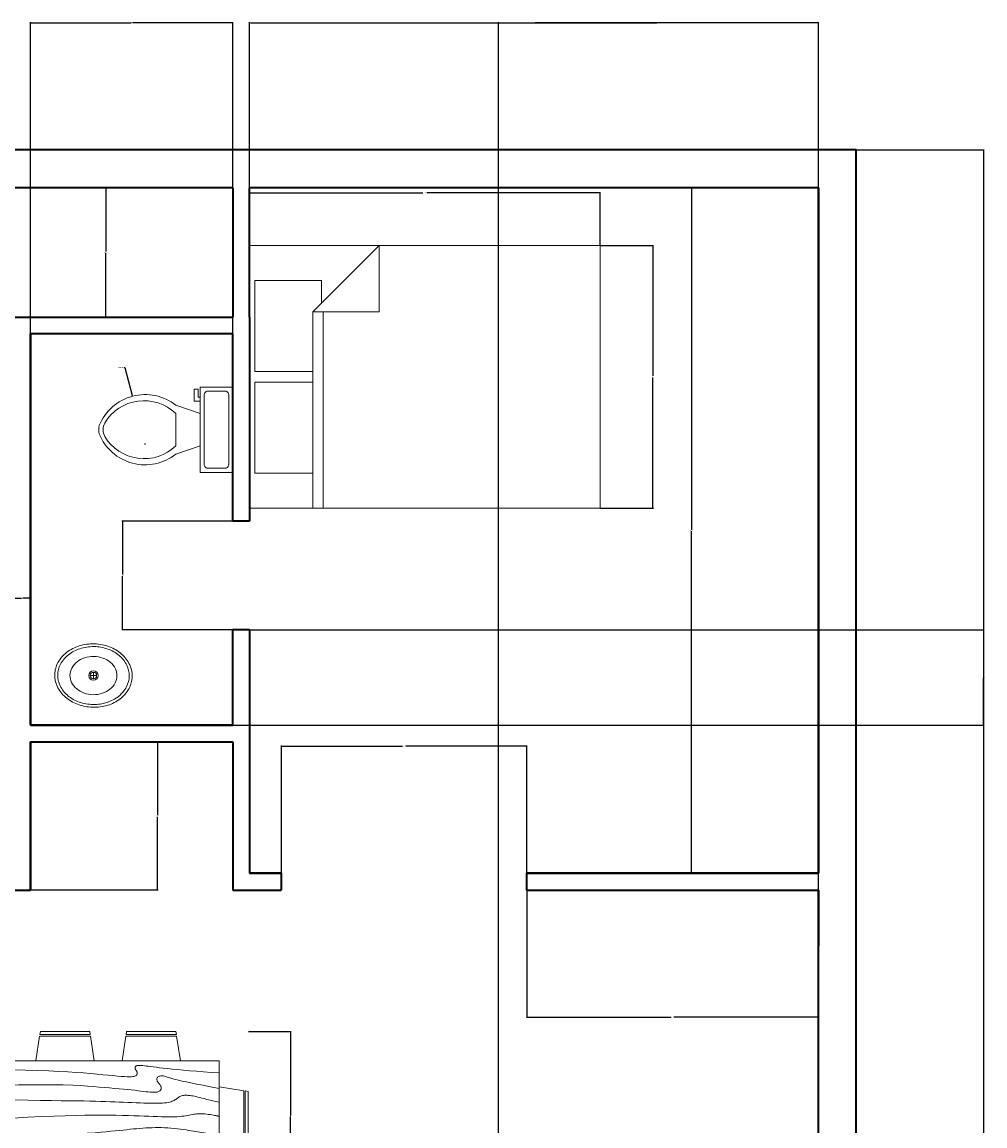
# Model space of a CAD drawing. Units: feet. Extents: x 2335 to 2876, y 491 to 1152.
# Tile 4 of 4: x 2648 to 2876, y 890 to 1152. Entities that reach past the tile are written whole.
import ezdxf

# ---------------------------------------------------------------- set-up
doc = ezdxf.new("R2010")
doc.units = ezdxf.units.FT
for name, color, linetype, lineweight in [('A-ANNO-DIMS', 2, 'Continuous', 18), ('A-FLOR-FIXT', 9, 'Continuous', 18), ('A-FURN', 8, 'Continuous', 18), ('A-WALL', 7, 'Continuous', 35), ('C-PROP', 3, 'Continuous', 35)]:
    doc.layers.add(name, color=color, linetype=linetype, lineweight=lineweight)
doc.styles.get("Standard").update_dxf_attribs({"font": 'arial.ttf'})
doc.dimstyles.get("Standard").update_dxf_attribs({"dimtxt": 0.18, "dimasz": 0.18, "dimexe": 0.18, "dimexo": 0.0625, "dimgap": 0.09, "dimtad": 0, "dimtih": 1, "dimtoh": 1, "dimdec": 4, "dimzin": 0, "dimdsep": 46, "dimlunit": 4, "dimtxsty": 'Standard', "dimcen": 0.09, "dimadec": 0, "dimazin": 0, "dimtfac": 1, "dimtdec": 4, "dimtofl": 0, "dimtmove": 0, "dimatfit": 3, "dimfxl": 1, "dimtolj": 1, "dimtzin": 0, "dimarcsym": 0})

# ---------------------------------------------------------------- blocks, each defined once
blk = doc.blocks.new('Bed - Queen')
for p, q in [((0, -80.00003), (0, 0)), ((0, 0), (59.99999, 0)), ((59.99999, 0), (59.99999, -80.00003)), ((7.99999, -1.2), (28.79998, -1.2)), ((7.99999, -14.4), (7.99999, -1.2)), ((28.79998, -1.2), (28.79998, -14.4)), ((31.19999, -1.2), (51.99999, -1.2)), ((31.19999, -14.4), (31.19999, -1.2)), ((51.99999, -1.2), (51.99999, -16.4)), ((0, -14.4), (44.8, -14.4)), ((59.99999, -29.6), (44.8, -14.4)), ((44.8, -14.4), (44.8, -29.6)), ((44.8, -16.8), (0, -16.8)), ((51.99999, -16.4), (46.79936, -16.4)), ((44.8, -29.6), (59.99999, -29.6)), ((59.99999, -80.00003), (0, -80.00003))]:
    blk.add_line(p, q)
blk = doc.blocks.new('Toilet - top')
for p, q in [((9.5, -6), (9.5, -2)), ((-8, -8.5), (-8, -8)), ((-7, -8), (-7, -9.5)), ((-4, -8), (-6, -14)), ((4, -8), (6, -14)), ((-10, -8.5), (-8, -8.5)), ((-10, -9.5), (-10, -8.5)), ((-7, -9.5), (-10, -9.5)), ((4, -14), (-4, -14))]:
    blk.add_line(p, q)
blk.add_lwpolyline([(10.5, -8), (10.5, 0), (-10.5, 0), (-10.5, -8)], close=True)
for points in [[(-9.5, -2), (-9.5, -6)], [(8.5, -1), (-8.5, -1)], [(-8.5, -7), (8.5, -7)]]:
    blk.add_lwpolyline(points)
for centre, radius, start, end in [((-8.62, -1.88), 0.884, 81.8699, 188.1301), ((8.62, -1.88), 0.884, 351.8699, 98.1301), ((-8.62, -6.12), 0.884, 171.8699, 278.1301), ((8.62, -6.12), 0.884, 261.8699, 8.1301), ((3.52, -21.58), 12.17, 141.4691, 247.9714), ((4.2, -21.82), 11.33, 136.3677, 238.9468), ((-3.52, -21.58), 12.17, 292.0284, 38.5307), ((-4.2, -21.82), 11.33, 301.053, 43.6321), ((0, -27.88), 4, 245.7318, 294.2682), ((0, -29), 4, 254.8605, 285.1395)]:
    blk.add_arc(centre, radius, start, end)
blk = doc.blocks.new('Sink - Oval top')
for p, q in [((-1, 0), (1, 0)), ((0, 1), (0, -1))]:
    blk.add_line(p, q)
for points in [[(-12.23, 0.39, 0.117634), (-11.46, -3.36, 0.104469), (-8.88, -6.8, 0.090016), (-5.08, -9.07, 0.08192), (-0.32, -10.02, 0.08192), (4.49, -9.38, 0.090016), (8.42, -7.36, 0.104469), (11.22, -4.09, 0.117634), (12.23, -0.39, 0.117634), (11.46, 3.36, 0.104469), (8.88, 6.8, 0.090016), (5.08, 9.07, 0.08192), (0.32, 10.02, 0.08192), (-4.49, 9.38, 0.090016), (-8.42, 7.36, 0.104469), (-11.22, 4.09, 0.117634)], [(-11.29, 0.16, 0.118622), (-10.52, -3.25, 0.104678), (-8.07, -6.36, 0.089562), (-4.54, -8.37, 0.081185), (-0.13, -9.15, 0.081185), (4.3, -8.49, 0.089562), (7.89, -6.58, 0.104678), (10.42, -3.55, 0.118622), (11.29, -0.16, 0.118622), (10.52, 3.25, 0.104678), (8.07, 6.36, 0.089562), (4.54, 8.37, 0.081185), (0.13, 9.15, 0.081185), (-4.3, 8.49, 0.089562), (-7.89, 6.58, 0.104678), (-10.42, 3.55, 0.118622)], [(-7.42, 0.08, 0.118283), (-6.91, -2.17, 0.104607), (-5.29, -4.21, 0.089718), (-2.97, -5.53, 0.081436), (-0.07, -6.04, 0.081436), (2.84, -5.59, 0.089718), (5.2, -4.33, 0.104607), (6.86, -2.32, 0.118283), (7.42, -0.08, 0.118283), (6.91, 2.17, 0.104607), (5.29, 4.21, 0.089718), (2.97, 5.53, 0.081436), (0.07, 6.04, 0.081436), (-2.84, 5.59, 0.089718), (-5.2, 4.33, 0.104607), (-6.86, 2.32, 0.118283)]]:
    blk.add_lwpolyline(points, format="xyb", close=True)
for radius in [1.5, 1]:
    blk.add_circle((0, 0), radius)
blk = doc.blocks.new('Dining Set - 36 x 72 in.')
for p, q in [((-22.2343, 26.00059), (-23.4847, 17.99762)), ((-22.2304, 26), (-5.7608, 26)), ((-22, 27.5), (-22.1562, 26.50042)), ((-5.8416, 26.5), (-22.1534, 26.5)), ((-22, 27.5), (-6, 27.5)), ((-5.8437, 26.49966), (-6, 27.5)), ((-4.5152, 17.99762), (-5.7655, 25.99926)), ((5.7657, 26.00059), (4.5153, 17.99762)), ((5.7696, 26), (22.2392, 26)), ((6, 27.5), (5.8438, 26.50042)), ((22.1584, 26.5), (5.8466, 26.5)), ((6, 27.5), (22, 27.5)), ((22.1563, 26.49966), (22, 27.5)), ((23.4848, 17.99762), (22.2345, 25.99926)), ((36, 18), (-36, 18)), ((-36, 18), (-36, -18)), ((36, -18), (36, 18)), ((-45.5, 8), (-44.5004, 8.15617)), ((-45.5, 8), (-45.5, -8)), ((-44.5, -8.15843), (-44.5, 8.15338)), ((-44.0006, 8.23428), (-35.9976, 9.48474)), ((-44, 8.23041), (-44, -8.23915)), ((44.0006, 8.23428), (35.9976, 9.48474)), ((44, 8.23041), (44, -8.23915)), ((44.5, -8.15843), (44.5, 8.15338)), ((45.5, 8), (44.5005, 8.15617)), ((45.5, 8), (45.5, -8)), ((-44.4997, -8.15631), (-45.5, -8)), ((-35.9976, -9.48476), (-43.9993, -8.2345)), ((35.9976, -9.48476), (43.9993, -8.2345)), ((44.4997, -8.15631), (45.5, -8)), ((-36, -18), (36, -18)), ((-22.2343, -26.0006), (-23.4847, -17.99762)), ((-4.5152, -17.99762), (-5.7655, -25.99928)), ((5.7657, -26.0006), (4.5153, -17.99762)), ((23.4848, -17.99762), (22.2345, -25.99928)), ((-22.2304, -26), (-5.7608, -26)), ((-22, -27.5), (-22.1562, -26.50044)), ((-5.8416, -26.5), (-22.1534, -26.5)), ((-22, -27.5), (-6, -27.5)), ((-5.8437, -26.49967), (-6, -27.5)), ((5.7696, -26), (22.2392, -26)), ((6, -27.5), (5.8438, -26.50044)), ((22.1584, -26.5), (5.8466, -26.5)), ((6, -27.5), (22, -27.5)), ((22.1563, -26.49967), (22, -27.5))]:
    blk.add_line(p, q)
for points in [[(-36, 15), (-31.1772, 14.97754), (-26.8079, 14.91406), (-22.8538, 14.81543), (-19.276, 14.6875), (-16.0362, 14.53613), (-13.0957, 14.36718), (-10.4159, 14.18652), (-7.9583, 14), (-5.6904, 13.81315), (-3.6035, 13.63021), (-1.6954, 13.45508), (0.0365, 13.29166), (1.5945, 13.14388), (2.9811, 13.01562), (4.1988, 12.9108), (5.25, 12.83333), (6.1393, 12.78613), (6.8802, 12.76823), (7.4883, 12.77767), (7.9792, 12.8125), (8.3685, 12.87077), (8.6719, 12.95052), (8.9049, 13.0498), (9.0833, 13.16666), (9.2205, 13.29899), (9.3216, 13.44401), (9.3895, 13.59879), (9.4271, 13.76041), (9.4373, 13.92594), (9.4232, 14.09245), (9.3875, 14.257), (9.3333, 14.41666), (9.2638, 14.56917), (9.1836, 14.71484), (9.0975, 14.85465), (9.0104, 14.98958), (8.9272, 15.1206), (8.8529, 15.2487), (8.7922, 15.37483), (8.75, 15.5), (8.7305, 15.62467), (8.7344, 15.74739), (8.7617, 15.86621), (8.8125, 15.97916), (8.8867, 16.08431), (8.9844, 16.17968), (9.1055, 16.26334), (9.25, 16.33333), (9.4189, 16.38802), (9.6172, 16.42708), (9.8506, 16.45052), (10.125, 16.45833), (10.4463, 16.45052), (10.8203, 16.42708), (11.2529, 16.38802), (11.75, 16.33333), (12.3184, 16.26318), (12.9694, 16.17838), (13.7151, 16.07991), (14.5677, 15.96875), (15.5395, 15.84586), (16.6426, 15.71224), (17.8893, 15.56884), (19.2917, 15.41666), (20.859, 15.25667), (22.5879, 15.08984), (24.4721, 14.91715), (26.5052, 14.73958), (28.6809, 14.5581), (30.9929, 14.3737), (33.4347, 14.18733), (36, 14)], [(-36, 10), (-28.9766, 10.14274), (-23.1725, 10.20442), (-18.4241, 10.19775), (-14.5677, 10.13541), (-11.4399, 10.03011), (-8.877, 9.89453), (-6.7154, 9.74137), (-4.7917, 9.58333), (-2.9698, 9.43082), (-1.2246, 9.28515), (0.4415, 9.14534), (2.026, 9.01041), (3.5266, 8.87939), (4.9408, 8.7513), (6.266, 8.62516), (7.5, 8.5), (8.6411, 8.37549), (9.6914, 8.2539), (10.6538, 8.13818), (11.5312, 8.03125), (12.3267, 7.93603), (13.043, 7.85547), (13.6831, 7.79248), (14.25, 7.75), (14.7471, 7.7303), (15.1797, 7.73307), (15.5537, 7.75732), (15.875, 7.80208), (16.1494, 7.86637), (16.3828, 7.94922), (16.5811, 8.04964), (16.75, 8.16666), (16.8944, 8.29915), (17.0143, 8.44531), (17.1089, 8.60319), (17.1771, 8.77083), (17.218, 8.94629), (17.2305, 9.1276), (17.2137, 9.31282), (17.1667, 9.5), (17.0895, 9.6875), (16.987, 9.875), (16.8649, 10.0625), (16.7292, 10.25), (16.5856, 10.4375), (16.4401, 10.625), (16.2985, 10.8125), (16.1667, 11), (16.05, 11.18733), (15.9518, 11.3737), (15.8752, 11.5581), (15.8229, 11.73958), (15.798, 11.91715), (15.8034, 12.08984), (15.842, 12.25667), (15.9167, 12.41666), (16.0295, 12.56836), (16.1784, 12.70833), (16.3605, 12.83268), (16.5729, 12.9375), (16.8127, 13.01888), (17.0768, 13.07291), (17.3625, 13.0957), (17.6667, 13.08333), (17.9894, 13.03312), (18.3418, 12.94726), (18.7382, 12.82918), (19.1927, 12.68229), (19.7195, 12.51001), (20.3327, 12.31575), (21.0465, 12.10294), (21.875, 11.875), (22.8357, 11.63354), (23.959, 11.37304), (25.2786, 11.08618), (26.8282, 10.76562), (28.6414, 10.40405), (30.752, 9.99414), (33.1936, 9.52856), (36, 9)], [(-36, 5.5), (-30.7157, 5.3348), (-26.069, 5.20963), (-21.9946, 5.11767), (-18.4271, 5.05208), (-15.3009, 5.00602), (-12.5508, 4.97265), (-10.1112, 4.94515), (-7.9167, 4.91666), (-5.909, 4.88167), (-4.0586, 4.83984), (-2.3429, 4.79215), (-0.7396, 4.73958), (0.7739, 4.6831), (2.22, 4.6237), (3.6213, 4.56233), (5, 4.5), (6.373, 4.43782), (7.7344, 4.3776), (9.0723, 4.32129), (10.375, 4.27083), (11.6309, 4.22819), (12.8281, 4.19531), (13.9551, 4.17415), (15, 4.16666), (15.954, 4.17448), (16.819, 4.19791), (17.6001, 4.23698), (18.3021, 4.29166), (18.9299, 4.36198), (19.4883, 4.44791), (19.9823, 4.54948), (20.4167, 4.66666), (20.7969, 4.79899), (21.1302, 4.94401), (21.4245, 5.09879), (21.6875, 5.26041), (21.9271, 5.42594), (22.1511, 5.59245), (22.3672, 5.757), (22.5834, 5.91666), (22.8065, 6.06868), (23.0404, 6.21093), (23.2879, 6.34147), (23.5521, 6.45833), (23.8358, 6.55957), (24.142, 6.64323), (24.4735, 6.70735), (24.8334, 6.75), (25.2235, 6.76969), (25.642, 6.76692), (26.0858, 6.74267), (26.5521, 6.69791), (27.0379, 6.63362), (27.5404, 6.55078), (28.0565, 6.45036), (28.5834, 6.33333), (29.1242, 6.19987), (29.7071, 6.04687), (30.3661, 5.87044), (31.1354, 5.66666), (32.0493, 5.43164), (33.142, 5.16146), (34.4475, 4.85221), (36, 4.5)], [(-36, -1), (-30.7915, -0.6591), (-26.0195, -0.38216), (-21.6519, -0.16284), (-17.6563, 0.00521), (-14.0005, 0.12833), (-10.6523, 0.21289), (-7.5796, 0.26522), (-4.75, 0.29166), (-2.134, 0.29793), (0.2878, 0.28711), (2.5317, 0.26163), (4.6146, 0.22396), (6.5529, 0.17651), (8.3633, 0.12174), (10.0623, 0.06209), (11.6667, 0), (13.1899, -0.06201), (14.6341, -0.1211), (15.9982, -0.17432), (17.2813, -0.21875), (18.4823, -0.25147), (19.6003, -0.26953), (20.6343, -0.27002), (21.5834, -0.25), (22.4481, -0.20768), (23.2357, -0.14584), (23.9549, -0.06836), (24.6146, 0.02083), (25.2235, 0.11784), (25.7904, 0.21875), (26.3241, 0.31966), (26.8334, 0.41666), (27.3265, 0.50618), (27.8099, 0.58593), (28.2894, 0.65397), (28.7709, 0.70833), (29.2601, 0.74707), (29.763, 0.76823), (30.2855, 0.76985), (30.8334, 0.75), (31.4088, 0.70784), (31.9994, 0.64713), (32.589, 0.57275), (33.1615, 0.48958), (33.7008, 0.4025), (34.1908, 0.3164), (34.6153, 0.23616), (34.9584, 0.16666), (35.2099, 0.11165), (35.3848, 0.07031), (35.504, 0.04069), (35.5886, 0.02083), (35.6594, 0.00879), (35.7377, 0.0026), (35.8442, 0.00032), (36, 0)], [(-36, -6.5), (-27.1843, -6.31267), (-20.084, -6.1263), (-14.469, -5.9419), (-10.1094, -5.76042), (-6.7752, -5.58285), (-4.2363, -5.41016), (-2.2629, -5.24333), (-0.625, -5.08334), (0.8708, -4.93099), (2.2715, -4.78646), (3.5872, -4.64974), (4.8281, -4.52084), (6.0046, -4.39974), (7.127, -4.28646), (8.2053, -4.18099), (9.25, -4.08334), (10.2705, -3.99382), (11.2734, -3.91407), (12.2647, -3.84603), (13.25, -3.79167), (14.2354, -3.75293), (15.2266, -3.73177), (16.2295, -3.73015), (17.25, -3.75), (18.2912, -3.79248), (19.3451, -3.85547), (20.4009, -3.93604), (21.4479, -4.03125), (22.4754, -4.13819), (23.4727, -4.25391), (24.4289, -4.37549), (25.3334, -4.5), (26.1785, -4.62492), (26.9694, -4.74935), (27.7145, -4.87281), (28.4219, -4.99479), (29.1, -5.11483), (29.7572, -5.23242), (30.4016, -5.34709), (31.0417, -5.45834), (31.6837, -5.56437), (32.3262, -5.65821), (32.9658, -5.73153), (33.599, -5.77604), (34.2224, -5.78345), (34.8327, -5.74545), (35.4264, -5.65373), (36, -5.5)], [(-36, -10), (-26.4022, -9.81299), (-18.4675, -9.62891), (-11.9839, -9.45069), (-6.7396, -9.28125), (-2.5226, -9.12354), (0.8789, -8.98047), (3.6769, -8.85498), (6.0833, -8.75), (8.2767, -8.66765), (10.3021, -8.60677), (12.1712, -8.56543), (13.8958, -8.54167), (15.4876, -8.53353), (16.9583, -8.53907), (18.3197, -8.55632), (19.5834, -8.58334), (20.7616, -8.61841), (21.8685, -8.66081), (22.9188, -8.71004), (23.9271, -8.76563), (24.9081, -8.82707), (25.8763, -8.89388), (26.8465, -8.96558), (27.8334, -9.04167), (28.8474, -9.12118), (29.8828, -9.20117), (30.93, -9.27824), (31.9792, -9.34896), (33.0205, -9.40991), (34.0443, -9.45768), (35.0407, -9.48885), (36, -9.5)], [(-36, -14.5), (-30.0881, -14.33513), (-25.0332, -14.21224), (-20.7312, -14.12647), (-17.0781, -14.07292), (-13.97, -14.04671), (-11.3027, -14.04297), (-8.9724, -14.05681), (-6.875, -14.08334), (-4.9224, -14.11833), (-3.0905, -14.16016), (-1.3709, -14.20785), (0.2448, -14.26042), (1.7647, -14.3169), (3.1973, -14.3763), (4.5507, -14.43767), (5.8333, -14.5), (7.0554, -14.5621), (8.235, -14.62175), (9.3922, -14.67652), (10.5469, -14.72396), (11.7192, -14.76164), (12.929, -14.78711), (14.1965, -14.79794), (15.5417, -14.79167), (16.9933, -14.76424), (18.6152, -14.70508), (20.4804, -14.60197), (22.6615, -14.44271), (25.2312, -14.21509), (28.2624, -13.9069), (31.8277, -13.50594), (36, -13)]]:
    blk.add_lwpolyline(points)
blk = doc.blocks.new('*D10')
at = {"layer": 'A-ANNO-DIMS', "color": 0, "lineweight": -2, "transparency": 16777216}
for p, q in [((2701.8, 1098.88), (2701.8, 1111.48)), ((2701.98, 1111.3), (2742.89, 1111.3)), ((2784.81, 1111.3), (2743.9, 1111.3)), ((2784.99, 1098.88), (2784.99, 1111.48))]:
    blk.add_line(p, q, dxfattribs=at)
at = {"layer": 'A-ANNO-DIMS', "color": 0, "transparency": 16777216}
for points in [[(2701.98, 1111.33), (2701.98, 1111.27), (2701.8, 1111.3)], [(2784.81, 1111.33), (2784.81, 1111.27), (2784.99, 1111.3)]]:
    blk.add_solid(points, dxfattribs=at)
at = {"layer": 'Defpoints', "color": 0, "transparency": 16777216}
for p in [(2701.8, 1111.3), (2701.8, 1098.82), (2784.99, 1098.82)]:
    blk.add_point(p, dxfattribs=at)
at = {"layer": 'A-ANNO-DIMS', "color": 0, "transparency": 16777216, "insert": (2743.4, 1111.3), "char_height": 0.18, "attachment_point": 5}
blk.add_mtext('\\A1;BED 83', dxfattribs=at)
blk = doc.blocks.new('*D11')
at = {"layer": 'A-ANNO-DIMS', "color": 0, "lineweight": -2, "transparency": 16777216}
for p, q in [((2785.06, 1098.82), (2797.65, 1098.82)), ((2797.47, 1098.64), (2797.47, 1067.81)), ((2797.47, 1036.6), (2797.47, 1067.44)), ((2785.06, 1036.42), (2797.65, 1036.42))]:
    blk.add_line(p, q, dxfattribs=at)
at = {"layer": 'A-ANNO-DIMS', "color": 0, "transparency": 16777216}
for points in [[(2797.44, 1098.64), (2797.5, 1098.64), (2797.47, 1098.82)], [(2797.44, 1036.6), (2797.5, 1036.6), (2797.47, 1036.42)]]:
    blk.add_solid(points, dxfattribs=at)
at = {"layer": 'Defpoints', "color": 0, "transparency": 16777216}
for p in [(2784.99, 1098.82), (2797.47, 1098.82), (2784.99, 1036.42)]:
    blk.add_point(p, dxfattribs=at)
at = {"layer": 'A-ANNO-DIMS', "color": 0, "transparency": 16777216, "insert": (2797.47, 1067.62), "char_height": 0.18, "attachment_point": 5}
blk.add_mtext('\\A1;62', dxfattribs=at)
blk = doc.blocks.new('*D21')
at = {"layer": 'A-ANNO-DIMS', "color": 0, "lineweight": -2, "transparency": 16777216}
for p, q in [((2701.56, 912.23), (2711.65, 912.23)), ((2711.47, 912.05), (2711.47, 892.31)), ((2711.47, 872.2), (2711.47, 891.94)), ((2701.56, 872.02), (2711.65, 872.02))]:
    blk.add_line(p, q, dxfattribs=at)
at = {"layer": 'A-ANNO-DIMS', "color": 0, "transparency": 16777216}
for points in [[(2711.44, 912.05), (2711.5, 912.05), (2711.47, 912.23)], [(2711.44, 872.2), (2711.5, 872.2), (2711.47, 872.02)]]:
    blk.add_solid(points, dxfattribs=at)
at = {"layer": 'Defpoints', "color": 0, "transparency": 16777216}
for p in [(2701.49, 912.23), (2711.47, 912.23), (2701.49, 872.02)]:
    blk.add_point(p, dxfattribs=at)
at = {"layer": 'A-ANNO-DIMS', "color": 0, "transparency": 16777216, "insert": (2711.47, 892.13), "char_height": 0.18, "attachment_point": 5}
blk.add_mtext('\\A1;40', dxfattribs=at)
blk = doc.blocks.new('*D25')
at = {"layer": 'A-ANNO-DIMS', "color": 0, "lineweight": -2, "transparency": 16777216}
for p, q in [((2845.86, 1121.49), (2876.13, 1121.49)), ((2875.95, 1121.31), (2875.95, 821.67)), ((2875.95, 521.67), (2875.95, 821.31)), ((2845.86, 521.49), (2876.13, 521.49))]:
    blk.add_line(p, q, dxfattribs=at)
at = {"layer": 'A-ANNO-DIMS', "color": 0, "transparency": 16777216}
for points in [[(2875.92, 1121.31), (2875.98, 1121.31), (2875.95, 1121.49)], [(2875.92, 521.67), (2875.98, 521.67), (2875.95, 521.49)]]:
    blk.add_solid(points, dxfattribs=at)
at = {"layer": 'Defpoints', "color": 0, "transparency": 16777216}
for p in [(2845.8, 1121.49), (2875.95, 1121.49), (2845.8, 521.49)]:
    blk.add_point(p, dxfattribs=at)
at = {"layer": 'A-ANNO-DIMS', "color": 0, "transparency": 16777216, "insert": (2875.95, 821.49), "char_height": 0.18, "attachment_point": 5}
blk.add_mtext('\\A1;600', dxfattribs=at)
blk = doc.blocks.new('*D36')
at = {"layer": 'A-ANNO-DIMS', "color": 0, "lineweight": -2, "transparency": 16777216}
for p, q in [((2836.73, 1112.49), (2806.47, 1112.49)), ((2806.65, 1112.31), (2806.65, 1031.32)), ((2806.65, 949.98), (2806.65, 1030.96)), ((2836.73, 949.8), (2806.47, 949.8))]:
    blk.add_line(p, q, dxfattribs=at)
at = {"layer": 'A-ANNO-DIMS', "color": 0, "transparency": 16777216}
for points in [[(2806.62, 1112.31), (2806.68, 1112.31), (2806.65, 1112.49)], [(2806.62, 949.98), (2806.68, 949.98), (2806.65, 949.8)]]:
    blk.add_solid(points, dxfattribs=at)
at = {"layer": 'Defpoints', "color": 0, "transparency": 16777216}
for p in [(2806.65, 1112.49), (2836.8, 1112.49), (2836.8, 949.8)]:
    blk.add_point(p, dxfattribs=at)
at = {"layer": 'A-ANNO-DIMS', "color": 0, "transparency": 16777216, "insert": (2806.65, 1031.14), "char_height": 0.18, "attachment_point": 5}
blk.add_mtext('\\A1;162.7', dxfattribs=at)
blk = doc.blocks.new('*D37')
at = {"layer": 'A-ANNO-DIMS', "color": 0, "lineweight": -2, "transparency": 16777216}
for p, q in [((2760.88, 882.29), (2760.88, 1151.82)), ((2761.06, 1151.64), (2798.45, 1151.64)), ((2836.62, 1151.64), (2799.23, 1151.64)), ((2836.8, 882.29), (2836.8, 1151.82))]:
    blk.add_line(p, q, dxfattribs=at)
at = {"layer": 'A-ANNO-DIMS', "color": 0, "transparency": 16777216}
for points in [[(2761.06, 1151.67), (2761.06, 1151.61), (2760.88, 1151.64)], [(2836.62, 1151.67), (2836.62, 1151.61), (2836.8, 1151.64)]]:
    blk.add_solid(points, dxfattribs=at)
at = {"layer": 'Defpoints', "color": 0, "transparency": 16777216}
for p in [(2836.8, 1151.64), (2760.88, 882.23), (2836.8, 882.23)]:
    blk.add_point(p, dxfattribs=at)
at = {"layer": 'A-ANNO-DIMS', "color": 0, "transparency": 16777216, "insert": (2798.84, 1151.64), "char_height": 0.18, "attachment_point": 5}
blk.add_mtext('\\A1;75.92', dxfattribs=at)
blk = doc.blocks.new('*D56')
at = {"layer": 'A-ANNO-DIMS', "color": 0, "lineweight": -2, "transparency": 16777216}
for p, q in [((2649.8, 1077.86), (2649.8, 1151.82)), ((2649.98, 1151.64), (2673.57, 1151.64)), ((2697.62, 1151.64), (2674.02, 1151.64)), ((2697.8, 1077.86), (2697.8, 1151.82))]:
    blk.add_line(p, q, dxfattribs=at)
at = {"layer": 'A-ANNO-DIMS', "color": 0, "transparency": 16777216}
for points in [[(2649.98, 1151.67), (2649.98, 1151.61), (2649.8, 1151.64)], [(2697.62, 1151.67), (2697.62, 1151.61), (2697.8, 1151.64)]]:
    blk.add_solid(points, dxfattribs=at)
at = {"layer": 'Defpoints', "color": 0, "transparency": 16777216}
for p in [(2697.8, 1151.64), (2649.8, 1077.8), (2697.8, 1077.8)]:
    blk.add_point(p, dxfattribs=at)
at = {"layer": 'A-ANNO-DIMS', "color": 0, "transparency": 16777216, "insert": (2673.8, 1151.64), "char_height": 0.18, "attachment_point": 5}
blk.add_mtext('\\A1;48', dxfattribs=at)
blk = doc.blocks.new('*D57')
at = {"layer": 'A-ANNO-DIMS', "color": 0, "lineweight": -2, "transparency": 16777216}
for p, q in [((2645.8, 985.02), (2645.8, 1015.28)), ((2645.98, 1015.1), (2647.65, 1015.1)), ((2649.62, 1015.1), (2647.95, 1015.1)), ((2649.8, 985.02), (2649.8, 1015.28))]:
    blk.add_line(p, q, dxfattribs=at)
at = {"layer": 'A-ANNO-DIMS', "color": 0, "transparency": 16777216}
for points in [[(2645.98, 1015.13), (2645.98, 1015.07), (2645.8, 1015.1)], [(2649.62, 1015.13), (2649.62, 1015.07), (2649.8, 1015.1)]]:
    blk.add_solid(points, dxfattribs=at)
at = {"layer": 'Defpoints', "color": 0, "transparency": 16777216}
for p in [(2649.8, 1015.1), (2645.8, 984.95), (2649.8, 984.95)]:
    blk.add_point(p, dxfattribs=at)
at = {"layer": 'A-ANNO-DIMS', "color": 0, "transparency": 16777216, "insert": (2647.8, 1015.1), "char_height": 0.18, "attachment_point": 5}
blk.add_mtext('\\A1;4', dxfattribs=at)
blk = doc.blocks.new('*D59')
at = {"layer": 'A-ANNO-DIMS', "color": 0, "lineweight": -2, "transparency": 16777216}
for p, q in [((2649.86, 980.95), (2680.13, 980.95)), ((2679.95, 980.77), (2679.95, 963.56)), ((2679.95, 945.98), (2679.95, 963.19)), ((2649.86, 945.8), (2680.13, 945.8))]:
    blk.add_line(p, q, dxfattribs=at)
at = {"layer": 'A-ANNO-DIMS', "color": 0, "transparency": 16777216}
for points in [[(2679.92, 980.77), (2679.98, 980.77), (2679.95, 980.95)], [(2679.92, 945.98), (2679.98, 945.98), (2679.95, 945.8)]]:
    blk.add_solid(points, dxfattribs=at)
at = {"layer": 'Defpoints', "color": 0, "transparency": 16777216}
for p in [(2649.8, 980.95), (2649.8, 945.8), (2679.95, 945.8)]:
    blk.add_point(p, dxfattribs=at)
at = {"layer": 'A-ANNO-DIMS', "color": 0, "transparency": 16777216, "insert": (2679.95, 963.38), "char_height": 0.18, "attachment_point": 5}
blk.add_mtext('\\A1;35.155', dxfattribs=at)
blk = doc.blocks.new('*D60')
at = {"layer": 'A-ANNO-DIMS', "color": 0, "lineweight": -2, "transparency": 16777216}
for p, q in [((2697.73, 1112.49), (2667.47, 1112.49)), ((2667.65, 1112.31), (2667.65, 1097.32)), ((2667.65, 1081.98), (2667.65, 1096.96)), ((2697.73, 1081.8), (2667.47, 1081.8))]:
    blk.add_line(p, q, dxfattribs=at)
at = {"layer": 'A-ANNO-DIMS', "color": 0, "transparency": 16777216}
for points in [[(2667.62, 1112.31), (2667.68, 1112.31), (2667.65, 1112.49)], [(2667.62, 1081.98), (2667.68, 1081.98), (2667.65, 1081.8)]]:
    blk.add_solid(points, dxfattribs=at)
at = {"layer": 'Defpoints', "color": 0, "transparency": 16777216}
for p in [(2667.65, 1112.49), (2697.8, 1112.49), (2697.8, 1081.8)]:
    blk.add_point(p, dxfattribs=at)
at = {"layer": 'A-ANNO-DIMS', "color": 0, "transparency": 16777216, "insert": (2667.65, 1097.14), "char_height": 0.18, "attachment_point": 5}
blk.add_mtext('\\A1;30.69', dxfattribs=at)
blk = doc.blocks.new('*D61')
at = {"layer": 'A-ANNO-DIMS', "color": 0, "lineweight": -2, "transparency": 16777216}
for p, q in [((2701.8, 1112.55), (2701.8, 1151.82)), ((2701.98, 1151.64), (2769.02, 1151.64)), ((2836.62, 1151.64), (2769.58, 1151.64)), ((2836.8, 1112.55), (2836.8, 1151.82))]:
    blk.add_line(p, q, dxfattribs=at)
at = {"layer": 'A-ANNO-DIMS', "color": 0, "transparency": 16777216}
for points in [[(2701.98, 1151.67), (2701.98, 1151.61), (2701.8, 1151.64)], [(2836.62, 1151.67), (2836.62, 1151.61), (2836.8, 1151.64)]]:
    blk.add_solid(points, dxfattribs=at)
at = {"layer": 'Defpoints', "color": 0, "transparency": 16777216}
for p in [(2836.8, 1151.64), (2701.8, 1112.49), (2836.8, 1112.49)]:
    blk.add_point(p, dxfattribs=at)
at = {"layer": 'A-ANNO-DIMS', "color": 0, "transparency": 16777216, "insert": (2769.3, 1151.64), "char_height": 0.18, "attachment_point": 5}
blk.add_mtext('\\A1;135', dxfattribs=at)
blk = doc.blocks.new('*D62')
at = {"layer": 'A-ANNO-DIMS', "color": 0, "lineweight": -2, "transparency": 16777216}
for p, q in [((2709.33, 949.86), (2709.33, 980.13)), ((2767.62, 949.86), (2767.62, 980.13)), ((2709.51, 979.95), (2738.08, 979.95)), ((2767.44, 979.95), (2738.87, 979.95))]:
    blk.add_line(p, q, dxfattribs=at)
at = {"layer": 'A-ANNO-DIMS', "color": 0, "transparency": 16777216}
for points in [[(2709.51, 979.98), (2709.51, 979.92), (2709.33, 979.95)], [(2767.44, 979.98), (2767.44, 979.92), (2767.62, 979.95)]]:
    blk.add_solid(points, dxfattribs=at)
at = {"layer": 'Defpoints', "color": 0, "transparency": 16777216}
for p in [(2767.62, 979.95), (2709.33, 949.8), (2767.62, 949.8)]:
    blk.add_point(p, dxfattribs=at)
at = {"layer": 'A-ANNO-DIMS', "color": 0, "transparency": 16777216, "insert": (2738.47, 979.95), "char_height": 0.18, "attachment_point": 5}
blk.add_mtext('\\A1;58.29', dxfattribs=at)
blk = doc.blocks.new('*D63')
at = {"layer": 'A-ANNO-DIMS', "color": 0, "lineweight": -2, "transparency": 16777216}
for p, q in [((2767.62, 945.74), (2767.62, 915.47)), ((2836.8, 945.74), (2836.8, 915.47)), ((2767.8, 915.65), (2801.81, 915.65)), ((2836.62, 915.65), (2802.6, 915.65))]:
    blk.add_line(p, q, dxfattribs=at)
at = {"layer": 'A-ANNO-DIMS', "color": 0, "transparency": 16777216}
for points in [[(2767.8, 915.68), (2767.8, 915.62), (2767.62, 915.65)], [(2836.62, 915.68), (2836.62, 915.62), (2836.8, 915.65)]]:
    blk.add_solid(points, dxfattribs=at)
at = {"layer": 'Defpoints', "color": 0, "transparency": 16777216}
for p in [(2767.62, 945.8), (2836.8, 945.8), (2767.62, 915.65)]:
    blk.add_point(p, dxfattribs=at)
at = {"layer": 'A-ANNO-DIMS', "color": 0, "transparency": 16777216, "insert": (2802.21, 915.65), "char_height": 0.18, "attachment_point": 5}
blk.add_mtext('\\A1;69.18', dxfattribs=at)
blk = doc.blocks.new('*D65')
at = {"layer": 'A-ANNO-DIMS', "color": 0, "lineweight": -2, "transparency": 16777216}
for p, q in [((2701.73, 1033.38), (2671.47, 1033.38)), ((2671.65, 1033.2), (2671.65, 1020.65)), ((2671.65, 1007.75), (2671.65, 1020.29)), ((2701.73, 1007.57), (2671.47, 1007.57))]:
    blk.add_line(p, q, dxfattribs=at)
at = {"layer": 'A-ANNO-DIMS', "color": 0, "transparency": 16777216}
for points in [[(2671.62, 1033.2), (2671.68, 1033.2), (2671.65, 1033.38)], [(2671.62, 1007.75), (2671.68, 1007.75), (2671.65, 1007.57)]]:
    blk.add_solid(points, dxfattribs=at)
at = {"layer": 'Defpoints', "color": 0, "transparency": 16777216}
for p in [(2671.65, 1033.38), (2701.8, 1033.38), (2701.8, 1007.57)]:
    blk.add_point(p, dxfattribs=at)
at = {"layer": 'A-ANNO-DIMS', "color": 0, "transparency": 16777216, "insert": (2671.65, 1020.47), "char_height": 0.18, "attachment_point": 5}
blk.add_mtext('\\A1;25.81', dxfattribs=at)
blk = doc.blocks.new('*D66')
at = {"layer": 'A-ANNO-DIMS', "color": 0, "lineweight": -2, "transparency": 16777216}
for p, q in [((2697.86, 1007.57), (2876.13, 1007.57)), ((2875.95, 1007.39), (2875.95, 996.44)), ((2875.95, 985.13), (2875.95, 996.08)), ((2697.86, 984.95), (2876.13, 984.95))]:
    blk.add_line(p, q, dxfattribs=at)
at = {"layer": 'A-ANNO-DIMS', "color": 0, "transparency": 16777216}
for points in [[(2875.92, 1007.39), (2875.98, 1007.39), (2875.95, 1007.57)], [(2875.92, 985.13), (2875.98, 985.13), (2875.95, 984.95)]]:
    blk.add_solid(points, dxfattribs=at)
at = {"layer": 'Defpoints', "color": 0, "transparency": 16777216}
for p in [(2697.8, 1007.57), (2875.95, 1007.57), (2697.8, 984.95)]:
    blk.add_point(p, dxfattribs=at)
at = {"layer": 'A-ANNO-DIMS', "color": 0, "transparency": 16777216, "insert": (2875.95, 996.26), "char_height": 0.18, "attachment_point": 5}
blk.add_mtext('\\A1;22.613', dxfattribs=at)
blk = doc.blocks.new('*D68')
at = {"layer": 'A-ANNO-DIMS', "color": 0, "lineweight": -2, "transparency": 16777216}
for p, q in [((2672.04, 1069.82), (2672.22, 1069.82)), ((2672.22, 1069.82), (2673.96, 1063.19)), ((2676.9, 1051.67), (2677.08, 1051.67)), ((2676.99, 1051.58), (2676.99, 1051.76))]:
    blk.add_line(p, q, dxfattribs=at)
at = {"layer": 'A-ANNO-DIMS', "color": 0, "transparency": 16777216}
blk.add_solid([(2673.99, 1063.2), (2673.94, 1063.18), (2674.01, 1063.02)], dxfattribs=at)
at = {"layer": 'Defpoints', "color": 0, "transparency": 16777216}
for p in [(2674.01, 1063.02), (2676.99, 1051.67)]:
    blk.add_point(p, dxfattribs=at)
at = {"layer": 'A-ANNO-DIMS', "color": 0, "transparency": 16777216, "insert": (2671.29, 1069.82), "char_height": 0.18, "attachment_point": 5}
blk.add_mtext('\\A1;4X R11.733', dxfattribs=at)

msp = doc.modelspace()

# ---------------------------------------------------------------- linework, layer by layer
at = {"layer": 'A-WALL'}
for p, q in [((2697.7974, 1112.4872), (2697.7974, 1081.7975)), ((2701.7974, 1081.7975), (2701.7974, 1112.4872)), ((2415.7974, 1081.7975), (2697.7974, 1081.7975)), ((2701.7974, 1081.7975), (2701.7974, 1033.3752)), ((2649.7974, 1077.7976), (2649.7974, 984.9529)), ((2649.7974, 1077.7976), (2649.7974, 984.9529)), ((2649.7974, 984.9529), (2649.7974, 1077.7976)), ((2697.7974, 1077.7975), (2649.7974, 1077.7976)), ((2697.7974, 1033.3752), (2697.7974, 1077.7975)), ((2701.7974, 1033.3752), (2697.7974, 1033.3752)), ((2697.7974, 984.9529), (2697.7974, 1007.5655)), ((2701.7974, 1007.5655), (2697.7974, 1007.5655)), ((2701.7974, 1007.5655), (2701.7974, 984.9529)), ((2697.7974, 984.9529), (2649.7974, 984.9529)), ((2697.7974, 984.9529), (2649.7974, 984.9529)), ((2649.7974, 984.9529), (2697.7974, 984.9529)), ((2649.7974, 984.9529), (2697.7974, 984.9529)), ((2701.7974, 984.9529), (2701.7974, 980.9529)), ((2649.7974, 980.9529), (2649.7974, 945.7975)), ((2649.7974, 945.7975), (2649.7974, 980.9529)), ((2649.7974, 980.9529), (2697.7974, 980.9529)), ((2649.7974, 980.9529), (2649.7974, 945.7975)), ((2649.7974, 980.9529), (2697.7974, 980.9529)), ((2649.7974, 980.9529), (2697.7974, 980.9529)), ((2697.7974, 980.9529), (2697.7974, 945.7975)), ((2701.7974, 982.2636), (2701.7974, 949.7975)), ((2701.7974, 980.9529), (2701.7974, 949.7975)), ((2701.7974, 949.7975), (2709.3268, 949.7975)), ((2701.7974, 949.7975), (2709.3268, 949.7975)), ((2709.3268, 949.7975), (2701.7974, 949.7975)), ((2709.3268, 949.7975), (2709.3268, 945.7975)), ((2836.7967, 949.7975), (2767.6197, 949.7975)), ((2767.6197, 945.7975), (2767.6197, 949.7975)), ((2767.6197, 949.7975), (2836.7967, 949.7975)), ((2645.7974, 945.7975), (2649.7974, 945.7975)), ((2697.7974, 945.7975), (2701.7974, 945.7975)), ((2701.7974, 945.7975), (2709.3268, 945.7975)), ((2767.6197, 945.7975), (2836.7967, 945.7975))]:
    msp.add_line(p, q, dxfattribs=at)
at = {"layer": 'C-PROP'}
for p, q in [((2836.7967, 1112.4872), (2836.7967, 949.7975)), ((2836.7967, 945.7975), (2836.7967, 932.4872))]:
    msp.add_line(p, q, dxfattribs=at)
msp.add_lwpolyline([(2845.7967, 521.4872), (2845.7967, 1121.4872), (2365.7967, 1121.4872), (2365.7967, 521.4872)], close=True, dxfattribs=at)
for points in [[(2697.7974, 1112.4872), (2374.7967, 1112.4872), (2374.7967, 530.4872), (2593.7974, 530.4872)], [(2836.7967, 949.7975), (2836.7967, 1112.4872), (2701.7974, 1112.4872)], [(2836.7967, 762.2261), (2836.7967, 945.7975)]]:
    msp.add_lwpolyline(points, dxfattribs=at)

# ---------------------------------------------------------------- block references
at = {"layer": 'A-FLOR-FIXT', "xscale": 0.9641315578102057, "yscale": 0.9641315578102057, "zscale": 0.9641315578102057, "rotation": 270}
msp.add_blockref('Toilet - top', (2697.7974, 1055.0608), dxfattribs=at)
at = {"layer": 'A-FLOR-FIXT', "xscale": 0.7514563269629554, "yscale": 0.7514563269629554, "zscale": 0.7514563269629554}
msp.add_blockref('Sink - Oval top', (2664.7437, 996.7007), dxfattribs=at)
at = {"layer": 'A-FURN', "xscale": 1.039951342731912, "yscale": 1.039951342731912, "zscale": 1.039951342731912, "rotation": 89.99999999999999}
msp.add_blockref('Bed - Queen', (2701.7974, 1036.4249), dxfattribs=at)
at = {"layer": 'A-FURN', "xscale": 0.7311477324397611, "yscale": 0.7311477324397611, "zscale": 0.7311477324397611}
msp.add_blockref('Dining Set - 36 x 72 in.', (2668.2264, 892.1257), dxfattribs=at)

# ---------------------------------------------------------------- dimensions: what is measured, and where the dimension line sits
at = {"layer": 'A-ANNO-DIMS'}
for base, p1, p2, override, picture, middle in [((2697.7974, 1151.6372), (2649.7974, 1077.7976), (2697.7974, 1077.7975), {"dimdec": 0, "dimlfac": 1, "dimrnd": 0, "dimzin": 0, "dimdsep": 46, "dimlunit": 2}, '*D56', (2673.7974, 1151.6372)), ((2836.7967, 1151.6372), (2701.7974, 1112.4872), (2836.7967, 1112.4872), {"dimdec": 0, "dimlfac": 1, "dimrnd": 0, "dimzin": 0, "dimdsep": 46, "dimlunit": 2}, '*D61', (2769.297, 1151.6372)), ((2836.7967, 1151.6372), (2760.8783, 882.2261), (2836.7967, 882.2261), {"dimdec": 2, "dimlfac": 1, "dimrnd": 0, "dimzin": 0, "dimdsep": 46, "dimlunit": 2}, '*D37', (2798.8375, 1151.6372)), ((2649.7974, 1015.1029), (2645.7974, 984.9529), (2649.7974, 984.9529), {"dimdec": 0, "dimlfac": 1, "dimrnd": 0, "dimzin": 0, "dimdsep": 46, "dimlunit": 2}, '*D57', (2647.7974, 1015.1029)), ((2767.6197, 979.9475), (2709.3268, 949.7975), (2767.6197, 949.7975), {"dimdec": 2, "dimlfac": 1, "dimrnd": 0, "dimzin": 0, "dimdsep": 46, "dimlunit": 2}, '*D62', (2738.4733, 979.9475))]:
    dim = msp.add_linear_dim(base=base, p1=p1, p2=p2, dimstyle='Standard', override=override, dxfattribs=at)
    dim.commit()
    dim.dimension.update_dxf_attribs({"geometry": picture, "text_midpoint": middle})
for base, p1, p2, angle, override, picture, middle in [((2875.9467, 1121.4872), (2845.7967, 521.4872), (2845.7967, 1121.4872), 90, {"dimdec": 0, "dimlfac": 1, "dimrnd": 0, "dimzin": 0, "dimdsep": 46, "dimlunit": 2}, '*D25', (2875.9467, 821.4872)), ((2667.6474, 1112.4872), (2697.7974, 1081.7975), (2697.7974, 1112.4872), 90, {"dimdec": 2, "dimlfac": 1, "dimrnd": 0, "dimzin": 0, "dimdsep": 46, "dimlunit": 2}, '*D60', (2667.6474, 1097.1423)), ((2806.6467, 1112.4872), (2836.7967, 949.7975), (2836.7967, 1112.4872), 90, {"dimdec": 1, "dimlfac": 1, "dimrnd": 0, "dimzin": 0, "dimdsep": 46, "dimlunit": 2}, '*D36', (2806.6467, 1031.1423)), ((2797.473, 1098.8219), (2784.9935, 1036.4249), (2784.9935, 1098.8219), 90, {"dimdec": 0, "dimlfac": 1, "dimrnd": 0, "dimzin": 0, "dimdsep": 46, "dimlunit": 2}, '*D11', (2797.473, 1067.6234)), ((2671.6474, 1033.3752), (2701.7974, 1007.5655), (2701.7974, 1033.3752), 90, {"dimdec": 2, "dimlfac": 1, "dimrnd": 0, "dimzin": 0, "dimdsep": 46, "dimlunit": 2}, '*D65', (2671.6474, 1020.4704)), ((2875.9467, 1007.5655), (2697.7974, 984.9529), (2697.7974, 1007.5655), 90, {"dimdec": 3, "dimlfac": 1, "dimrnd": 0, "dimzin": 0, "dimdsep": 46, "dimlunit": 2}, '*D66', (2875.9467, 996.2592)), ((2679.9474, 945.7975), (2649.7974, 980.9529), (2649.7974, 945.7975), 270, {"dimdec": 3, "dimlfac": 1, "dimrnd": 0, "dimzin": 0, "dimdsep": 46, "dimlunit": 2}, '*D59', (2679.9474, 963.3752)), ((2767.6197, 915.6475), (2836.7967, 945.7975), (2767.6197, 945.7975), 180, {"dimdec": 2, "dimlfac": 1, "dimrnd": 0, "dimzin": 0, "dimdsep": 46, "dimlunit": 2}, '*D63', (2802.2082, 915.6475)), ((2711.4738, 912.2323), (2701.4936, 872.0191), (2701.4936, 912.2323), 90, {"dimdec": 0, "dimlfac": 1, "dimrnd": 0, "dimzin": 0, "dimdsep": 46, "dimlunit": 2}, '*D21', (2711.4738, 892.1257))]:
    dim = msp.add_linear_dim(base=base, p1=p1, p2=p2, angle=angle, dimstyle='Standard', override=override, dxfattribs=at)
    dim.commit()
    dim.dimension.update_dxf_attribs({"geometry": picture, "text_midpoint": middle})
dim = msp.add_linear_dim(base=(2701.7974, 1111.3013), p1=(2784.9935, 1098.8219), p2=(2701.7974, 1098.8219), angle=180, text='BED <>', dimstyle='Standard', override={"dimdec": 0, "dimlfac": 1, "dimrnd": 0, "dimzin": 0, "dimdsep": 46, "dimlunit": 2}, dxfattribs=at)
dim.commit()
dim.dimension.update_dxf_attribs({"geometry": '*D10', "text_midpoint": (2743.3955, 1111.3013)})
dim = msp.add_radius_dim(center=(2676.991, 1051.6675), mpoint=(2674.01, 1063.015), text='4X <>', dimstyle='Standard', override={"dimdec": 3, "dimlfac": 1, "dimrnd": 0, "dimzin": 0, "dimdsep": 46, "dimlunit": 2}, dxfattribs=at)
dim.commit()
dim.dimension.update_dxf_attribs({"geometry": '*D68', "text_midpoint": (2671.2947, 1069.8235), "dimtype": 164})

doc.saveas('drawing.dxf')
